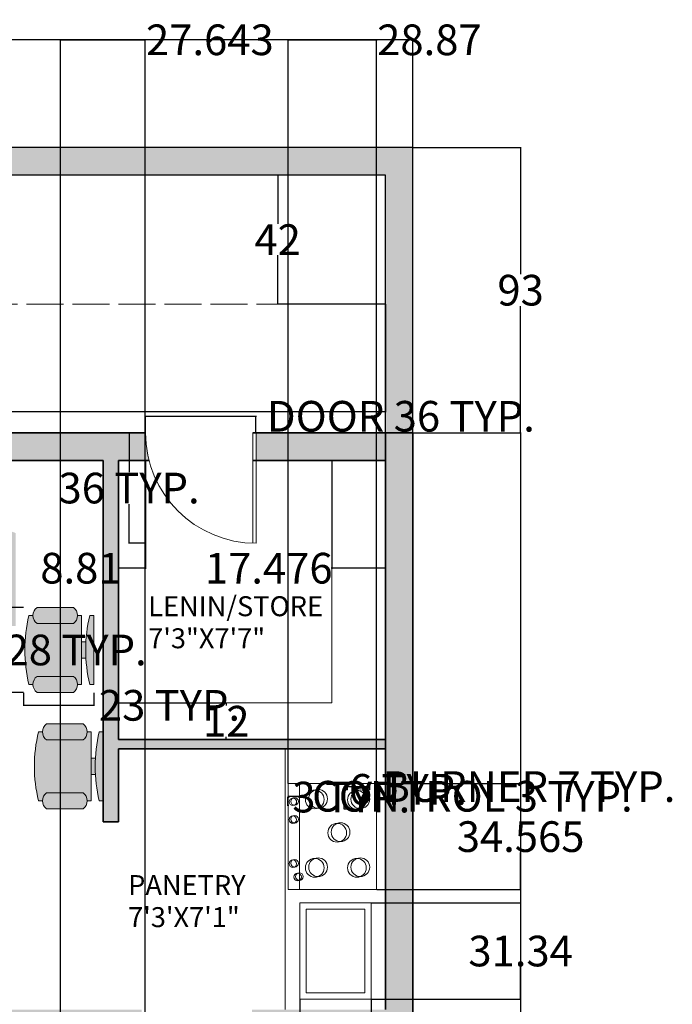
# Model space of a CAD drawing. Units: inches. Extents: x 409 to 1056, y 160 to 945.
# Tile 6 of 6: x 843 to 1056, y 624 to 945. Entities that reach past the tile are written whole.
import ezdxf

# ---------------------------------------------------------------- set-up
doc = ezdxf.new("R2010")
doc.units = ezdxf.units.IN
doc.header["$MEASUREMENT"] = 0
doc.linetypes.add('ACAD_ISO02W100', pattern=[15, 12, -3])
for name, color, linetype, lineweight in [('A-ANNO-DIMS', 2, 'Continuous', 18), ('A-AREA-IDEN', 7, 'Continuous', 18), ('A-DOOR', 3, 'Continuous', 18), ('A-EQPM', 8, 'Continuous', 18), ('A-FLOR-CASE', 8, 'Continuous', 20), ('A-FLOR-FIXT', 8, 'Continuous', 18), ('A-FURN', 8, 'Continuous', 18), ('A-ROOF-BYND', 8, 'ACAD_ISO02W100', 13), ('A-WALL', 7, 'Continuous', 35), ('A-WALL-PRPT', 7, 'Continuous', 30)]:
    doc.layers.add(name, color=color, linetype=linetype, lineweight=lineweight)
doc.layers.add('A-FURN-PATT', color=51, linetype='Continuous', lineweight=13, true_color=0xf8f6b0)
doc.layers.add('A-WALL-PATT', color=251, linetype='Continuous', lineweight=13, true_color=0x636466)
doc.styles.get("Standard").update_dxf_attribs({"font": 'arial.ttf'})
doc.dimstyles.get("Standard").update_dxf_attribs({"dimtxt": 10, "dimasz": 0.18, "dimexe": 0.18, "dimexo": 0.0625, "dimgap": 0.09, "dimtad": 0, "dimtih": 1, "dimtoh": 1, "dimdec": 0, "dimzin": 0, "dimdsep": 46, "dimlunit": 3, "dimtxsty": 'Standard', "dimcen": 0.09, "dimadec": 0, "dimazin": 0, "dimtfac": 1, "dimtdec": 0, "dimtofl": 0, "dimtmove": 0, "dimatfit": 3, "dimfxl": 1, "dimtolj": 1, "dimtzin": 0, "dimarcsym": 0})

# ---------------------------------------------------------------- blocks, each defined once
blk = doc.blocks.new('Chair - Desk')
for p, q in [((-8.5, 0), (-8.5, -1)), ((-8.5, 0), (8.5, 0)), ((8.5, 0), (8.5, -1)), ((-2, -3), (-2, -1.9355)), ((2, -1.9576), (2, -3)), ((-8.5, -3), (-8.5, -4)), ((-8.5, -3), (8.5, -3)), ((8.5, -3), (8.5, -4)), ((-10.5, -5), (-10.5, -14)), ((-6.5, -14), (-6.5, -5)), ((6.5, -5), (6.5, -14)), ((10.5, -14), (10.5, -5)), ((-8.5, -15), (-8.5, -16)), ((8.5, -15), (8.5, -16))]:
    blk.add_line(p, q)
for centre, radius, start, end in [((0, 34.625), 36.625, 256.5803, 283.4197), ((-8.5, -6.5), 2.5, 36.8699, 143.1301), ((8.5, -6.5), 2.5, 36.8699, 143.1301), ((-8.5, -12.5), 2.5, 216.8699, 323.1301), ((8.5, -12.5), 2.5, 216.8699, 323.1301), ((0, 19.625), 36.625, 256.5803, 283.4197)]:
    blk.add_arc(centre, radius, start, end)
blk = doc.blocks.new('DOOR-SWING-36IN')
for p, q in [((35, 36), (35, 0)), ((36, 36), (36, 0))]:
    blk.add_line(p, q)
blk.add_arc((36, 36), 36, 180, 270)
blk = doc.blocks.new('COOKTOP-BURNER')
for centre in [(3.06, 3.06), (4.16, 3.26)]:
    blk.add_circle(centre, 3.06)
blk = doc.blocks.new('COOKTOP-CONTROL')
for centre in [(1.22, 1.22), (1.79, 1.36)]:
    blk.add_circle(centre, 1.22)
blk = doc.blocks.new('*D11')
at = {"layer": 'A-ANNO-DIMS', "color": 0, "lineweight": -2, "transparency": 16777216}
for p, q in [((884.55, 810.81), (884.55, 816.32)), ((884.73, 816.14), (920.37, 816.14)), ((920.55, 810.81), (920.55, 816.32)), ((920.55, 816.14), (920.73, 816.14))]:
    blk.add_line(p, q, dxfattribs=at)
at = {"layer": 'A-ANNO-DIMS', "color": 0, "transparency": 16777216}
for points in [[(884.73, 816.17), (884.73, 816.11), (884.55, 816.14)], [(920.37, 816.17), (920.37, 816.11), (920.55, 816.14)]]:
    blk.add_solid(points, dxfattribs=at)
at = {"layer": 'Defpoints', "color": 0, "transparency": 16777216}
for p in [(920.55, 816.14), (884.55, 810.74), (920.55, 810.74)]:
    blk.add_point(p, dxfattribs=at)
at = {"layer": 'A-ANNO-DIMS', "color": 0, "transparency": 16777216, "insert": (967.81, 816.14), "char_height": 10, "attachment_point": 5}
blk.add_mtext('\\A1;DOOR 36 TYP.', dxfattribs=at)
blk = doc.blocks.new('*D12')
at = {"layer": 'A-ANNO-DIMS', "color": 0, "lineweight": -2, "transparency": 16777216}
for p, q in [((884.49, 810.74), (878.97, 810.74)), ((879.15, 810.56), (879.15, 797.94)), ((879.15, 774.92), (879.15, 787.54)), ((884.49, 774.74), (878.97, 774.74))]:
    blk.add_line(p, q, dxfattribs=at)
at = {"layer": 'A-ANNO-DIMS', "color": 0, "transparency": 16777216}
for points in [[(879.12, 810.56), (879.18, 810.56), (879.15, 810.74)], [(879.12, 774.92), (879.18, 774.92), (879.15, 774.74)]]:
    blk.add_solid(points, dxfattribs=at)
at = {"layer": 'Defpoints', "color": 0, "transparency": 16777216}
for p in [(879.15, 810.74), (884.55, 810.74), (884.55, 774.74)]:
    blk.add_point(p, dxfattribs=at)
at = {"layer": 'A-ANNO-DIMS', "color": 0, "transparency": 16777216, "insert": (879.15, 792.74), "char_height": 10, "attachment_point": 5}
blk.add_mtext('\\A1;36 TYP.', dxfattribs=at)
blk = doc.blocks.new('*D19')
at = {"layer": 'A-ANNO-DIMS', "color": 0, "lineweight": -2, "transparency": 16777216}
for p, q in [((844.66, 753.84), (840.37, 753.84)), ((840.55, 753.66), (840.55, 745.22)), ((840.55, 726.25), (840.55, 734.7)), ((844.66, 726.07), (840.37, 726.07))]:
    blk.add_line(p, q, dxfattribs=at)
at = {"layer": 'A-ANNO-DIMS', "color": 0, "transparency": 16777216}
for points in [[(840.52, 753.66), (840.58, 753.66), (840.55, 753.84)], [(840.52, 726.25), (840.58, 726.25), (840.55, 726.07)]]:
    blk.add_solid(points, dxfattribs=at)
at = {"layer": 'Defpoints', "color": 0, "transparency": 16777216}
for p in [(844.72, 753.84), (840.55, 726.07), (844.72, 726.07)]:
    blk.add_point(p, dxfattribs=at)
at = {"layer": 'A-ANNO-DIMS', "color": 0, "transparency": 16777216, "insert": (840.55, 739.96), "char_height": 10, "attachment_point": 5}
blk.add_mtext('\\A1;CHAIR 28 TYP.', dxfattribs=at)
blk = doc.blocks.new('*D20')
at = {"layer": 'A-ANNO-DIMS', "color": 0, "lineweight": -2, "transparency": 16777216}
for p, q in [((844.72, 726.01), (844.72, 721.73)), ((867.64, 726.01), (867.64, 721.73)), ((844.9, 721.91), (867.46, 721.91)), ((867.64, 721.91), (867.82, 721.91))]:
    blk.add_line(p, q, dxfattribs=at)
at = {"layer": 'A-ANNO-DIMS', "color": 0, "transparency": 16777216}
for points in [[(844.9, 721.94), (844.9, 721.88), (844.72, 721.91)], [(867.46, 721.94), (867.46, 721.88), (867.64, 721.91)]]:
    blk.add_solid(points, dxfattribs=at)
at = {"layer": 'Defpoints', "color": 0, "transparency": 16777216}
for p in [(844.72, 726.07), (867.64, 726.07), (867.64, 721.91)]:
    blk.add_point(p, dxfattribs=at)
at = {"layer": 'A-ANNO-DIMS', "color": 0, "transparency": 16777216, "insert": (892.33, 721.91), "char_height": 10, "attachment_point": 5}
blk.add_mtext('\\A1;23 TYP.', dxfattribs=at)
blk = doc.blocks.new('*D31')
at = {"layer": 'A-ANNO-DIMS', "color": 0, "lineweight": -2, "transparency": 16777216}
for p, q in [((950.42, 694.4), (950.42, 695.6)), ((950.6, 695.42), (957.46, 695.42)), ((957.64, 694.4), (957.64, 695.6)), ((957.64, 695.42), (957.82, 695.42))]:
    blk.add_line(p, q, dxfattribs=at)
at = {"layer": 'A-ANNO-DIMS', "color": 0, "transparency": 16777216}
for points in [[(950.6, 695.45), (950.6, 695.39), (950.42, 695.42)], [(957.46, 695.45), (957.46, 695.39), (957.64, 695.42)]]:
    blk.add_solid(points, dxfattribs=at)
at = {"layer": 'Defpoints', "color": 0, "transparency": 16777216}
for p in [(950.42, 694.34), (957.64, 695.42), (957.64, 694.34)]:
    blk.add_point(p, dxfattribs=at)
at = {"layer": 'A-ANNO-DIMS', "color": 0, "transparency": 16777216, "insert": (1009.57, 695.42), "char_height": 10, "attachment_point": 5}
blk.add_mtext('\\A1;BURNER 7 TYP.', dxfattribs=at)
blk = doc.blocks.new('*D32')
at = {"layer": 'A-ANNO-DIMS', "color": 0, "lineweight": -2, "transparency": 16777216}
for p, q in [((950.35, 694.34), (949.15, 694.34)), ((949.33, 694.34), (949.33, 694.52)), ((949.33, 694.52), (949.51, 694.52)), ((949.33, 688.2), (949.33, 694.16)), ((950.35, 688.02), (949.15, 688.02))]:
    blk.add_line(p, q, dxfattribs=at)
at = {"layer": 'A-ANNO-DIMS', "color": 0, "transparency": 16777216}
for points in [[(949.3, 694.16), (949.36, 694.16), (949.33, 694.34)], [(949.3, 688.2), (949.36, 688.2), (949.33, 688.02)]]:
    blk.add_solid(points, dxfattribs=at)
at = {"layer": 'Defpoints', "color": 0, "transparency": 16777216}
for p in [(949.33, 694.34), (950.42, 694.34), (950.42, 688.02)]:
    blk.add_point(p, dxfattribs=at)
at = {"layer": 'A-ANNO-DIMS', "color": 0, "transparency": 16777216, "insert": (970.08, 694.52), "char_height": 10, "attachment_point": 5}
blk.add_mtext('\\A1;6 TYP.', dxfattribs=at)
blk = doc.blocks.new('*D33')
at = {"layer": 'A-ANNO-DIMS', "color": 0, "lineweight": -2, "transparency": 16777216}
for p, q in [((931.36, 691.88), (931.36, 692.45)), ((931.54, 692.27), (934.2, 692.27)), ((934.38, 691.88), (934.38, 692.45)), ((934.38, 692.27), (934.56, 692.27))]:
    blk.add_line(p, q, dxfattribs=at)
at = {"layer": 'A-ANNO-DIMS', "color": 0, "transparency": 16777216}
for points in [[(931.54, 692.3), (931.54, 692.24), (931.36, 692.27)], [(934.2, 692.3), (934.2, 692.24), (934.38, 692.27)]]:
    blk.add_solid(points, dxfattribs=at)
at = {"layer": 'Defpoints', "color": 0, "transparency": 16777216}
for p in [(931.36, 691.82), (934.38, 692.27), (934.38, 691.82)]:
    blk.add_point(p, dxfattribs=at)
at = {"layer": 'A-ANNO-DIMS', "color": 0, "transparency": 16777216, "insert": (991.14, 692.27), "char_height": 10, "attachment_point": 5}
blk.add_mtext('\\A1;CONTROL 3 TYP.', dxfattribs=at)
blk = doc.blocks.new('*D34')
at = {"layer": 'A-ANNO-DIMS', "color": 0, "lineweight": -2, "transparency": 16777216}
for p, q in [((931.3, 691.82), (930.73, 691.82)), ((930.91, 691.82), (930.91, 692)), ((930.91, 692), (931.09, 692)), ((930.91, 689.41), (930.91, 691.64)), ((931.3, 689.23), (930.73, 689.23))]:
    blk.add_line(p, q, dxfattribs=at)
at = {"layer": 'A-ANNO-DIMS', "color": 0, "transparency": 16777216}
for points in [[(930.88, 691.64), (930.94, 691.64), (930.91, 691.82)], [(930.88, 689.41), (930.94, 689.41), (930.91, 689.23)]]:
    blk.add_solid(points, dxfattribs=at)
at = {"layer": 'Defpoints', "color": 0, "transparency": 16777216}
for p in [(930.91, 691.82), (931.36, 691.82), (931.36, 689.23)]:
    blk.add_point(p, dxfattribs=at)
at = {"layer": 'A-ANNO-DIMS', "color": 0, "transparency": 16777216, "insert": (951.63, 692), "char_height": 10, "attachment_point": 5}
blk.add_mtext('\\A1;3 TYP.', dxfattribs=at)
blk = doc.blocks.new('*D35')
at = {"layer": 'A-ANNO-DIMS', "color": 0, "lineweight": -2, "transparency": 16777216}
for p, q in [((455.74, 903.81), (455.74, 939.05)), ((455.92, 938.87), (702.61, 938.87)), ((971.56, 938.87), (724.88, 938.87)), ((971.74, 903.81), (971.74, 939.05))]:
    blk.add_line(p, q, dxfattribs=at)
at = {"layer": 'A-ANNO-DIMS', "color": 0, "transparency": 16777216}
for points in [[(455.92, 938.9), (455.92, 938.84), (455.74, 938.87)], [(971.56, 938.9), (971.56, 938.84), (971.74, 938.87)]]:
    blk.add_solid(points, dxfattribs=at)
at = {"layer": 'Defpoints', "color": 0, "transparency": 16777216}
for p in [(971.74, 938.87), (455.74, 903.74), (971.74, 903.74)]:
    blk.add_point(p, dxfattribs=at)
at = {"layer": 'A-ANNO-DIMS', "color": 0, "transparency": 16777216, "insert": (713.74, 938.87), "char_height": 10, "attachment_point": 5}
blk.add_mtext('\\A1;516', dxfattribs=at)
blk = doc.blocks.new('*D38')
at = {"layer": 'A-ANNO-DIMS', "color": 0, "lineweight": -2, "transparency": 16777216}
for p, q in [((971.8, 810.74), (1007.05, 810.74)), ((1006.87, 810.56), (1006.87, 530.94)), ((1006.87, 240.92), (1006.87, 520.55)), ((971.8, 240.74), (1007.05, 240.74))]:
    blk.add_line(p, q, dxfattribs=at)
at = {"layer": 'A-ANNO-DIMS', "color": 0, "transparency": 16777216}
for points in [[(1006.84, 810.56), (1006.9, 810.56), (1006.87, 810.74)], [(1006.84, 240.92), (1006.9, 240.92), (1006.87, 240.74)]]:
    blk.add_solid(points, dxfattribs=at)
at = {"layer": 'Defpoints', "color": 0, "transparency": 16777216}
for p in [(971.74, 810.74), (1006.87, 810.74), (971.74, 240.74)]:
    blk.add_point(p, dxfattribs=at)
at = {"layer": 'A-ANNO-DIMS', "color": 0, "transparency": 16777216, "insert": (1006.87, 525.74), "char_height": 10, "attachment_point": 5}
blk.add_mtext('\\A1;570', dxfattribs=at)
blk = doc.blocks.new('*D41')
at = {"layer": 'A-ANNO-DIMS', "color": 0, "lineweight": -2, "transparency": 16777216}
for p, q in [((934.87, 626.08), (934.87, 166.44)), ((958.09, 626.08), (958.09, 166.44)), ((935.05, 166.62), (957.91, 166.62)), ((958.09, 166.62), (958.27, 166.62))]:
    blk.add_line(p, q, dxfattribs=at)
at = {"layer": 'A-ANNO-DIMS', "color": 0, "transparency": 16777216}
for points in [[(935.05, 166.65), (935.05, 166.59), (934.87, 166.62)], [(957.91, 166.65), (957.91, 166.59), (958.09, 166.62)]]:
    blk.add_solid(points, dxfattribs=at)
at = {"layer": 'Defpoints', "color": 0, "transparency": 16777216}
for p in [(934.87, 626.14), (958.09, 626.14), (958.09, 166.62)]:
    blk.add_point(p, dxfattribs=at)
at = {"layer": 'A-ANNO-DIMS', "color": 0, "transparency": 16777216, "insert": (975.27, 166.62), "char_height": 10, "attachment_point": 5}
blk.add_mtext('\\A1;23.22', dxfattribs=at)
blk = doc.blocks.new('*D42')
at = {"layer": 'A-ANNO-DIMS', "color": 0, "lineweight": -2, "transparency": 16777216}
for p, q in [((958.15, 657.48), (1007.05, 657.48)), ((1006.87, 657.3), (1006.87, 647.01)), ((1006.87, 626.32), (1006.87, 636.61)), ((958.15, 626.14), (1007.05, 626.14))]:
    blk.add_line(p, q, dxfattribs=at)
at = {"layer": 'A-ANNO-DIMS', "color": 0, "transparency": 16777216}
for points in [[(1006.84, 657.3), (1006.9, 657.3), (1006.87, 657.48)], [(1006.84, 626.32), (1006.9, 626.32), (1006.87, 626.14)]]:
    blk.add_solid(points, dxfattribs=at)
at = {"layer": 'Defpoints', "color": 0, "transparency": 16777216}
for p in [(958.09, 657.48), (1006.87, 657.48), (958.09, 626.14)]:
    blk.add_point(p, dxfattribs=at)
at = {"layer": 'A-ANNO-DIMS', "color": 0, "transparency": 16777216, "insert": (1006.87, 641.81), "char_height": 10, "attachment_point": 5}
blk.add_mtext('\\A1;31.34', dxfattribs=at)
blk = doc.blocks.new('*D43')
at = {"layer": 'A-ANNO-DIMS', "color": 0, "lineweight": -2, "transparency": 16777216}
for p, q in [((931.02, 696.45), (931.02, 939.05)), ((931.2, 938.87), (959.71, 938.87)), ((959.89, 696.45), (959.89, 939.05)), ((959.89, 938.87), (960.07, 938.87))]:
    blk.add_line(p, q, dxfattribs=at)
at = {"layer": 'A-ANNO-DIMS', "color": 0, "transparency": 16777216}
for points in [[(931.2, 938.9), (931.2, 938.84), (931.02, 938.87)], [(959.71, 938.9), (959.71, 938.84), (959.89, 938.87)]]:
    blk.add_solid(points, dxfattribs=at)
at = {"layer": 'Defpoints', "color": 0, "transparency": 16777216}
for p in [(959.89, 938.87), (931.02, 696.39), (959.89, 696.39)]:
    blk.add_point(p, dxfattribs=at)
at = {"layer": 'A-ANNO-DIMS', "color": 0, "transparency": 16777216, "insert": (977.12, 938.87), "char_height": 10, "attachment_point": 5}
blk.add_mtext('\\A1;28.87', dxfattribs=at)
blk = doc.blocks.new('*D44')
at = {"layer": 'A-ANNO-DIMS', "color": 0, "lineweight": -2, "transparency": 16777216}
for p, q in [((959.95, 696.39), (1007.05, 696.39)), ((1006.87, 696.21), (1006.87, 684.31)), ((1006.87, 662), (1006.87, 673.91)), ((959.95, 661.82), (1007.05, 661.82))]:
    blk.add_line(p, q, dxfattribs=at)
at = {"layer": 'A-ANNO-DIMS', "color": 0, "transparency": 16777216}
for points in [[(1006.84, 696.21), (1006.9, 696.21), (1006.87, 696.39)], [(1006.84, 662), (1006.9, 662), (1006.87, 661.82)]]:
    blk.add_solid(points, dxfattribs=at)
at = {"layer": 'Defpoints', "color": 0, "transparency": 16777216}
for p in [(959.89, 696.39), (1006.87, 696.39), (959.89, 661.82)]:
    blk.add_point(p, dxfattribs=at)
at = {"layer": 'A-ANNO-DIMS', "color": 0, "transparency": 16777216, "insert": (1006.87, 679.11), "char_height": 10, "attachment_point": 5}
blk.add_mtext('\\A1;34.565', dxfattribs=at)
blk = doc.blocks.new('*D51')
at = {"layer": 'A-ANNO-DIMS', "color": 0, "lineweight": -2, "transparency": 16777216}
for p, q in [((856.74, 613.81), (856.74, 939.05)), ((856.92, 938.87), (884.2, 938.87)), ((884.38, 613.81), (884.38, 939.05)), ((884.38, 938.87), (884.56, 938.87))]:
    blk.add_line(p, q, dxfattribs=at)
at = {"layer": 'A-ANNO-DIMS', "color": 0, "transparency": 16777216}
for points in [[(856.92, 938.9), (856.92, 938.84), (856.74, 938.87)], [(884.2, 938.9), (884.2, 938.84), (884.38, 938.87)]]:
    blk.add_solid(points, dxfattribs=at)
at = {"layer": 'Defpoints', "color": 0, "transparency": 16777216}
for p in [(884.38, 938.87), (856.74, 613.74), (884.38, 613.74)]:
    blk.add_point(p, dxfattribs=at)
at = {"layer": 'A-ANNO-DIMS', "color": 0, "transparency": 16777216, "insert": (905.5, 938.87), "char_height": 10, "attachment_point": 5}
blk.add_mtext('\\A1;27.643', dxfattribs=at)
blk = doc.blocks.new('*D57')
at = {"layer": 'A-ANNO-DIMS', "color": 0, "lineweight": -2, "transparency": 16777216}
for p, q in [((875.74, 801.68), (875.74, 766.44)), ((884.55, 801.68), (884.55, 766.44)), ((875.74, 766.62), (875.56, 766.62)), ((884.37, 766.62), (875.92, 766.62))]:
    blk.add_line(p, q, dxfattribs=at)
at = {"layer": 'A-ANNO-DIMS', "color": 0, "transparency": 16777216}
for points in [[(875.92, 766.65), (875.92, 766.59), (875.74, 766.62)], [(884.37, 766.65), (884.37, 766.59), (884.55, 766.62)]]:
    blk.add_solid(points, dxfattribs=at)
at = {"layer": 'Defpoints', "color": 0, "transparency": 16777216}
for p in [(875.74, 801.74), (884.55, 801.74), (875.74, 766.62)]:
    blk.add_point(p, dxfattribs=at)
at = {"layer": 'A-ANNO-DIMS', "color": 0, "transparency": 16777216, "insert": (863.44, 766.62), "char_height": 10, "attachment_point": 5}
blk.add_mtext('\\A1;8.81', dxfattribs=at)
blk = doc.blocks.new('*D59')
at = {"layer": 'A-ANNO-DIMS', "color": 0, "lineweight": -2, "transparency": 16777216}
for p, q in [((971.8, 903.74), (1007.05, 903.74)), ((1006.87, 903.56), (1006.87, 862.44)), ((1006.87, 810.92), (1006.87, 852.04)), ((971.8, 810.74), (1007.05, 810.74))]:
    blk.add_line(p, q, dxfattribs=at)
at = {"layer": 'A-ANNO-DIMS', "color": 0, "transparency": 16777216}
for points in [[(1006.84, 903.56), (1006.9, 903.56), (1006.87, 903.74)], [(1006.84, 810.92), (1006.9, 810.92), (1006.87, 810.74)]]:
    blk.add_solid(points, dxfattribs=at)
at = {"layer": 'Defpoints', "color": 0, "transparency": 16777216}
for p in [(971.74, 903.74), (1006.87, 903.74), (971.74, 810.74)]:
    blk.add_point(p, dxfattribs=at)
at = {"layer": 'A-ANNO-DIMS', "color": 0, "transparency": 16777216, "insert": (1006.87, 857.24), "char_height": 10, "attachment_point": 5}
blk.add_mtext('\\A1;93', dxfattribs=at)
blk = doc.blocks.new('*D60')
at = {"layer": 'A-ANNO-DIMS', "color": 0, "lineweight": -2, "transparency": 16777216}
for p, q in [((537.3, 852.68), (537.3, 817.44)), ((962.74, 852.68), (962.74, 817.44)), ((537.48, 817.62), (728.99, 817.62)), ((962.56, 817.62), (771.05, 817.62))]:
    blk.add_line(p, q, dxfattribs=at)
at = {"layer": 'A-ANNO-DIMS', "color": 0, "transparency": 16777216}
for points in [[(537.48, 817.65), (537.48, 817.59), (537.3, 817.62)], [(962.56, 817.65), (962.56, 817.59), (962.74, 817.62)]]:
    blk.add_solid(points, dxfattribs=at)
at = {"layer": 'Defpoints', "color": 0, "transparency": 16777216}
for p in [(537.3, 852.74), (962.74, 852.74), (537.3, 817.62)]:
    blk.add_point(p, dxfattribs=at)
at = {"layer": 'A-ANNO-DIMS', "color": 0, "transparency": 16777216, "insert": (750.02, 817.62), "char_height": 10, "attachment_point": 5}
blk.add_mtext('\\A1;425.44', dxfattribs=at)
blk = doc.blocks.new('*D61')
at = {"layer": 'A-ANNO-DIMS', "color": 0, "lineweight": -2, "transparency": 16777216}
for p, q in [((962.68, 894.74), (927.44, 894.74)), ((927.62, 894.56), (927.62, 878.85)), ((927.62, 852.92), (927.62, 868.63)), ((962.68, 852.74), (927.44, 852.74))]:
    blk.add_line(p, q, dxfattribs=at)
at = {"layer": 'A-ANNO-DIMS', "color": 0, "transparency": 16777216}
for points in [[(927.59, 894.56), (927.65, 894.56), (927.62, 894.74)], [(927.59, 852.92), (927.65, 852.92), (927.62, 852.74)]]:
    blk.add_solid(points, dxfattribs=at)
at = {"layer": 'Defpoints', "color": 0, "transparency": 16777216}
for p in [(927.62, 894.74), (962.74, 894.74), (962.74, 852.74)]:
    blk.add_point(p, dxfattribs=at)
at = {"layer": 'A-ANNO-DIMS', "color": 0, "transparency": 16777216, "insert": (927.62, 873.74), "char_height": 10, "attachment_point": 5}
blk.add_mtext('\\A1;42', dxfattribs=at)
blk = doc.blocks.new('*D64')
at = {"layer": 'A-ANNO-DIMS', "color": 0, "lineweight": -2, "transparency": 16777216}
for p, q in [((945.27, 801.68), (945.27, 766.44)), ((962.74, 801.68), (962.74, 766.44)), ((945.27, 766.62), (945.09, 766.62)), ((962.56, 766.62), (945.45, 766.62))]:
    blk.add_line(p, q, dxfattribs=at)
at = {"layer": 'A-ANNO-DIMS', "color": 0, "transparency": 16777216}
for points in [[(945.45, 766.65), (945.45, 766.59), (945.27, 766.62)], [(962.56, 766.65), (962.56, 766.59), (962.74, 766.62)]]:
    blk.add_solid(points, dxfattribs=at)
at = {"layer": 'Defpoints', "color": 0, "transparency": 16777216}
for p in [(945.27, 801.74), (962.74, 801.74), (945.27, 766.62)]:
    blk.add_point(p, dxfattribs=at)
at = {"layer": 'A-ANNO-DIMS', "color": 0, "transparency": 16777216, "insert": (924.71, 766.62), "char_height": 10, "attachment_point": 5}
blk.add_mtext('\\A1;17.476', dxfattribs=at)
blk = doc.blocks.new('*D65')
at = {"layer": 'A-ANNO-DIMS', "color": 0, "lineweight": -2, "transparency": 16777216}
for p, q in [((875.8, 722.74), (911.05, 722.74)), ((910.87, 722.56), (910.87, 721.85)), ((875.8, 710.74), (911.05, 710.74)), ((910.87, 710.92), (910.87, 711.63))]:
    blk.add_line(p, q, dxfattribs=at)
at = {"layer": 'A-ANNO-DIMS', "color": 0, "transparency": 16777216}
for points in [[(910.84, 722.56), (910.9, 722.56), (910.87, 722.74)], [(910.84, 710.92), (910.9, 710.92), (910.87, 710.74)]]:
    blk.add_solid(points, dxfattribs=at)
at = {"layer": 'Defpoints', "color": 0, "transparency": 16777216}
for p in [(875.74, 722.74), (875.74, 710.74), (910.87, 710.74)]:
    blk.add_point(p, dxfattribs=at)
at = {"layer": 'A-ANNO-DIMS', "color": 0, "transparency": 16777216, "insert": (910.87, 716.74), "char_height": 10, "attachment_point": 5}
blk.add_mtext('\\A1;12', dxfattribs=at)

msp = doc.modelspace()

# ---------------------------------------------------------------- hatches: boundary and pattern name
at = {"layer": 'A-FURN-PATT', "transparency": 33554661}
h = msp.add_hatch(color=256, dxfattribs=at)
h.dxf.hatch_style = 1
h.paths.add_polyline_path([(700.0326, 771.7872), (672.0783, 771.7872), (672.0783, 749.5866), (700.0326, 749.5866)], flags=17)
h.paths.add_polyline_path([(727.9869, 771.7872), (700.0326, 771.7872), (700.0326, 749.5866), (727.9869, 749.5866)], flags=17)
h.paths.add_polyline_path([(700.0326, 779.6917), (700.0326, 771.7872), (727.9869, 771.7872), (727.9869, 774.0139, 0.05064665)], flags=17)
h.paths.add_polyline_path([(700.0326, 779.6917, 0.04962821), (672.0783, 779.6917), (672.0783, 771.7872), (700.0326, 771.7872)], flags=17)
h.paths.add_polyline_path([(672.0783, 779.6917, 0.05064665), (644.124, 774.0139), (644.124, 771.7872), (672.0783, 771.7872)], flags=17)
h.paths.add_polyline_path([(672.0783, 771.7872), (644.124, 771.7872), (644.124, 749.5866), (672.0783, 749.5866)], flags=17)
h.paths.add_polyline_path([(637.1355, 778.0558), (637.1355, 747.772), (644.124, 747.772), (644.124, 774.0139, -0.15194781), (727.9869, 774.0139), (727.9869, 771.7872), (727.9869, 749.5866), (727.9869, 747.772), (734.9755, 747.772), (734.9755, 778.0558, 0.19047621)])
h.paths.add_polyline_path([(751.3563, 774.0139, -0.15194781), (835.2192, 774.0139), (835.2192, 747.772), (842.2077, 747.772), (842.2077, 778.0558, 0.19047621), (744.3677, 778.0558), (744.3677, 747.772), (751.3563, 747.772)])
h.paths.add_polyline_path([(779.3105, 771.7872), (751.3563, 771.7872), (751.3563, 749.5866), (779.3106, 749.5866)], flags=17)
h.paths.add_polyline_path([(807.2649, 771.7872), (779.3105, 771.7872), (779.3106, 749.5866), (807.2648, 749.5866)], flags=17)
h.paths.add_polyline_path([(835.2192, 771.7872), (807.2649, 771.7872), (807.2648, 749.5866), (835.2192, 749.5866)], flags=17)
h.paths.add_polyline_path([(835.2192, 774.0139, 0.05064665), (807.2649, 779.6917), (807.2649, 771.7872), (835.2192, 771.7872)], flags=17)
h.paths.add_polyline_path([(807.2649, 779.6917, 0.04962821), (779.3105, 779.6917), (779.3105, 771.7872), (807.2649, 771.7872)], flags=17)
h.paths.add_polyline_path([(779.3105, 779.6917, 0.05064665), (751.3563, 774.0139), (751.3563, 771.7872), (779.3105, 771.7872)], flags=17)
h.paths.add_polyline_path([(863.6721, 751.196), (862.3498, 751.196, -0.23606798), (861.0276, 748.5515), (849.1271, 748.5515, -0.23606798), (847.8048, 751.196), (846.4825, 751.196, 0.11764706), (846.4825, 728.7174), (847.8048, 728.7174, -0.23606798), (849.1271, 731.3619), (861.0276, 731.3619, -0.23606798), (862.3498, 728.7174), (863.6721, 728.7174)])
h.paths.add_polyline_path([(861.0276, 753.8406), (849.1271, 753.8406, 0.5), (849.1271, 748.5515), (861.0276, 748.5515, 0.23606798), (862.3498, 751.196, 0.23606798)])
h.paths.add_polyline_path([(861.0276, 731.3619), (849.1271, 731.3619, 0.23606798), (847.8048, 728.7174, 0.23606798), (849.1271, 726.0728), (861.0276, 726.0728, 0.5)])
h.paths.add_polyline_path([(867.6389, 751.196), (866.3167, 751.196, 0.11764706), (866.3167, 728.7174), (867.6389, 728.7174)])
h.paths.add_polyline_path([(865.0666, 742.6012), (863.6721, 742.6012), (863.6721, 737.3121), (865.0666, 737.3121, -0.02732414)])
h.paths.add_polyline_path([(864.1304, 715.9038), (852.2299, 715.9038, 0.5), (852.2299, 710.6147), (864.1304, 710.6147, 0.5)])
h.paths.add_polyline_path([(866.7749, 713.2593), (865.4527, 713.2593, -0.23606798), (864.1304, 710.6147), (852.2299, 710.6147, -0.23606798), (850.9076, 713.2593), (849.5854, 713.2593, 0.11764706), (849.5854, 690.7806), (850.9076, 690.7806, -0.23606798), (852.2299, 693.4252), (864.1304, 693.4252, -0.23606798), (865.4527, 690.7806), (866.7749, 690.7806)])
h.paths.add_polyline_path([(864.1304, 693.4252), (852.2299, 693.4252, 0.5), (852.2299, 688.1361), (864.1304, 688.1361, 0.5)])
h.paths.add_polyline_path([(868.1695, 704.6645), (866.7749, 704.6645), (866.7749, 699.3754), (868.1695, 699.3754, -0.02732414)])
h.paths.add_polyline_path([(870.7418, 713.2593), (869.4195, 713.2593, 0.11764706), (869.4195, 690.7806), (870.7418, 690.7806)])
h.paths.add_polyline_path([(796.1541, 700.7668), (803.8768, 698.1956), (796.8278, 694.1258, 4.66316556)])
h.paths.add_polyline_path([(722.7253, 700.7668), (730.4481, 698.1956), (723.399, 694.1258, 4.66316556)])
h.paths.add_polyline_path([(669.7198, 709.3627), (668.8708, 710.3764, -0.23606798), (665.9944, 709.692), (658.3533, 718.8153, -0.23606798), (659.5316, 721.527), (658.6826, 722.5407), (641.4498, 708.1074), (642.2988, 707.0937, -0.23606798), (645.1752, 707.7781), (652.8164, 698.6548, -0.23606798), (651.638, 695.9431), (652.487, 694.9294, 0.11764706)])
h.paths.add_polyline_path([(645.1752, 707.7781, 0.5), (641.1204, 704.382), (648.7616, 695.2587, 0.5), (652.8164, 698.6548)])
h.paths.add_polyline_path([(662.4081, 722.2113, 0.5), (658.3533, 718.8153), (665.9944, 709.692, 0.23606798), (668.8708, 710.3764, 0.23606798), (670.0492, 713.0881)])
h.paths.add_polyline_path([(656.9846, 724.5681), (656.1356, 725.5818), (638.9027, 711.1485), (639.7518, 710.1348, 0.11764706)])
h.paths.add_polyline_path([(652.0936, 717.0221), (651.1982, 718.0912, -0.02732414), (647.1434, 714.6951), (648.0388, 713.626)], flags=17)
at = {"layer": 'A-WALL-PATT'}
h = msp.add_hatch(color=256, dxfattribs=at)
h.dxf.hatch_style = 1
h.paths.add_polyline_path([(730.4481, 698.1956), (696.9841, 709.3369, 1), (696.9841, 678.8752)], flags=17)
h.paths.add_polyline_path([(803.8768, 698.1956), (770.4128, 709.3369, 1), (770.4128, 678.8752)], flags=17)
h.paths.add_polyline_path([(464.7418, 894.7439), (466.7418, 894.7439), (962.7418, 894.7439), (962.7418, 810.7439), (971.7418, 810.7439), (971.7418, 903.7439), (455.7418, 903.7439), (455.7418, 201.7439), (971.7418, 201.7439), (971.7418, 240.7439), (962.7418, 240.7439), (962.7418, 210.7439), (464.7418, 210.7439)])
h = msp.add_hatch(color=256, dxfattribs=at)
h.dxf.hatch_style = 1
h.paths.add_polyline_path([(626.7418, 801.7439), (870.7418, 801.7439), (870.7418, 710.7439), (870.7418, 683.9043), (875.7418, 683.9043), (875.7418, 707.7439), (962.7418, 707.7439), (962.7418, 710.7439), (875.7418, 710.7439), (875.7418, 722.7439), (875.7418, 801.7439), (885.6955, 801.7439, -0.06325422), (884.5523, 810.7439), (617.7418, 810.7439), (617.7418, 732.9297), (626.7418, 732.9297)])
h.paths.add_polyline_path([(962.7418, 810.7439), (920.5523, 810.7439), (920.5523, 801.7439), (962.7418, 801.7439)], flags=17)
h.paths.add_polyline_path([(971.7418, 810.7439), (962.7418, 810.7439), (962.7418, 801.7439), (962.7418, 707.7439), (962.7418, 622.7439), (962.7418, 613.7439), (962.7418, 548.7439), (856.7418, 548.7439), (847.7418, 548.7439), (776.7418, 548.7439), (776.7418, 569.8172), (768.7418, 569.8172), (768.7418, 539.7439), (847.7418, 539.7439), (971.7418, 539.7439), (971.7418, 613.7439), (971.7418, 707.7439)])
h.paths.add_polyline_path([(883.2418, 622.7439), (875.7418, 622.7439), (684.4993, 622.7439, -0.06325422), (685.6424, 613.7439), (870.7418, 613.7439), (875.7418, 613.7439), (884.3849, 613.7439, -0.06325422)])
h.paths.add_polyline_path([(649.6424, 622.7439), (626.7418, 622.7439), (626.7418, 613.7439), (649.6424, 613.7439)])
h.paths.add_polyline_path([(626.7418, 652.3165), (617.7418, 652.3165), (617.7418, 613.7439), (626.7418, 613.7439), (626.7418, 622.7439)])
h.paths.add_polyline_path([(776.7418, 613.7439), (768.7418, 613.7439), (768.7418, 590.4138), (776.7418, 590.4138)], flags=17)
h.paths.add_polyline_path([(856.7418, 613.7439), (847.7418, 613.7439), (847.7418, 548.7439), (856.7418, 548.7439)], flags=17)
h.paths.add_polyline_path([(962.7418, 622.7439), (919.2418, 622.7439), (919.2418, 613.7439), (962.7418, 613.7439)], flags=17)
h.paths.add_polyline_path([(971.7418, 539.7439), (962.7418, 539.7439), (962.7418, 452.7439), (687.1506, 452.7439, -0.06325422), (686.0074, 443.7439), (962.7418, 443.7439), (962.7418, 331.7439), (927.6873, 331.7439, -0.02784244), (927.9102, 327.7439), (962.7418, 327.7439), (962.7418, 249.7439), (871.7418, 249.7439), (870.7418, 249.7439), (626.7418, 249.7439), (626.7418, 282.7439), (617.7418, 282.7439), (617.7418, 240.7439), (870.7418, 240.7439), (871.7418, 240.7439), (971.7418, 240.7439), (971.7418, 249.7439), (971.7418, 327.7439), (971.7418, 331.7439), (971.7418, 443.7439), (971.7418, 452.7439)])
h.paths.add_polyline_path([(875.7418, 443.7439), (870.7418, 443.7439), (870.7418, 327.7439), (871.7418, 327.7439), (891.9102, 327.7439), (891.9102, 331.7439), (875.7418, 331.7439)], flags=17)

# ---------------------------------------------------------------- linework, layer by layer
at = {"layer": 'A-DOOR'}
for p, q in [((920.5523, 801.7439), (920.5523, 810.7439)), ((884.5523, 801.7439), (885.6955, 801.7439)), ((919.5523, 801.7439), (920.5523, 801.7439))]:
    msp.add_line(p, q, dxfattribs=at)
at = {"layer": 'A-EQPM'}
for p, q in [((931.0176, 661.8238), (931.0176, 696.3886)), ((931.0176, 696.3886), (934.7013, 696.3886)), ((934.7013, 661.8238), (931.0176, 661.8238))]:
    msp.add_line(p, q, dxfattribs=at)
msp.add_lwpolyline([(934.7013, 696.3886), (959.8882, 696.3886), (959.8882, 661.8238), (934.7013, 661.8238)], close=True, dxfattribs=at)
msp.add_circle((932.5858, 690.4505), 1.2239, dxfattribs=at)
at = {"layer": 'A-FLOR-CASE'}
for p, q in [((945.2662, 722.7439), (945.2662, 801.7439)), ((875.7418, 710.7439), (875.7418, 722.7439)), ((875.7418, 722.7439), (945.2662, 722.7439)), ((930.0665, 707.7439), (930.0665, 622.7439))]:
    msp.add_line(p, q, dxfattribs=at)
at = {"layer": 'A-FLOR-FIXT'}
for points in [[(934.8736, 657.4805), (958.0915, 657.4805), (958.0915, 626.1427), (934.8736, 626.1427)], [(936.8736, 655.4805), (956.0915, 655.4805), (956.0915, 628.1427), (936.8736, 628.1427)]]:
    msp.add_lwpolyline(points, close=True, dxfattribs=at)
at = {"layer": 'A-ROOF-BYND'}
msp.add_line((962.7418, 852.7439), (537.2978, 852.7439), dxfattribs=at)
at = {"layer": 'A-WALL'}
for p, q in [((884.5523, 810.7439), (617.7418, 810.7439)), ((884.5523, 810.7439), (875.7418, 810.7439)), ((971.7418, 810.7439), (919.5523, 810.7439)), ((971.7418, 810.7439), (919.5523, 810.7439)), ((962.7418, 801.7439), (962.7418, 810.7439)), ((971.7418, 705.7439), (971.7418, 810.7439)), ((870.7418, 801.7439), (626.7418, 801.7439)), ((870.7418, 801.7439), (870.7418, 710.7439)), ((875.7418, 801.7439), (875.7418, 710.7439)), ((885.6955, 801.7439), (875.7418, 801.7439)), ((962.7418, 801.7439), (919.5523, 801.7439)), ((962.7418, 707.7439), (962.7418, 801.7439)), ((870.7418, 683.9043), (870.7418, 710.7439)), ((875.7418, 710.7439), (962.7418, 710.7439)), ((875.7418, 707.7439), (875.7418, 683.9043)), ((875.7418, 707.7439), (962.7418, 707.7439)), ((962.7418, 707.7439), (962.7418, 622.7439)), ((971.7418, 707.7439), (971.7418, 613.7439)), ((870.7418, 683.9043), (875.7418, 683.9043))]:
    msp.add_line(p, q, dxfattribs=at)
at = {"layer": 'A-WALL-PRPT'}
for p, q in [((971.7418, 903.7439), (455.7418, 903.7439)), ((971.7418, 810.7439), (971.7418, 903.7439)), ((962.7418, 894.7439), (466.7418, 894.7439)), ((962.7418, 810.7439), (962.7418, 894.7439))]:
    msp.add_line(p, q, dxfattribs=at)

# ---------------------------------------------------------------- block references
at = {"layer": 'A-DOOR'}
msp.add_blockref('DOOR-SWING-36IN', (884.552, 774.744), dxfattribs=at)
at = {"layer": 'A-EQPM'}
for name, p in [('COOKTOP-BURNER', (936.6471, 688.1634)), ('COOKTOP-BURNER', (950.415, 688.018)), ('COOKTOP-CONTROL', (931.362, 689.227)), ('COOKTOP-CONTROL', (931.362, 683.4121)), ('COOKTOP-BURNER', (943.9771, 677.3024)), ('COOKTOP-CONTROL', (931.362, 669.06)), ('COOKTOP-BURNER', (936.6471, 665.8782)), ('COOKTOP-BURNER', (950.415, 665.8782)), ('COOKTOP-CONTROL', (932.9069, 664.7275))]:
    msp.add_blockref(name, p, dxfattribs=at)
at = {"layer": 'A-FURN', "xscale": 1.322274350512926, "yscale": 1.322274350512926, "zscale": 1.322274350512926, "rotation": 270}
for p in [(867.6389, 739.9567), (870.7418, 702.02)]:
    msp.add_blockref('Chair - Desk', p, dxfattribs=at)

# ---------------------------------------------------------------- texts
at = {"layer": 'A-AREA-IDEN'}
for s, height, p in [('LENIN/STORE', 6.506154, (885.3938, 750.9664)), ('7\'3"X7\'7"', 6.50615, (885.3938, 740.5148)), ('PANETRY', 6.50615, (878.8472, 660.0622)), ('7\'3\'X7\'1"', 6.50615, (878.8472, 649.6106))]:
    msp.add_text(s, height=height, dxfattribs=at).set_placement(p)

# ---------------------------------------------------------------- dimensions: what is measured, and where the dimension line sits
at = {"layer": 'A-ANNO-DIMS'}
for base, p1, p2, override, picture, middle in [((971.7418, 938.8689), (455.7418, 903.7439), (971.7418, 903.7439), {"dimdec": 0, "dimlfac": 1, "dimrnd": 0, "dimzin": 0, "dimdsep": 46, "dimlunit": 2}, '*D35', (713.7418, 938.8689)), ((884.3849, 938.8689), (856.7418, 613.7439), (884.3849, 613.7439), {"dimdec": 3, "dimlfac": 1, "dimrnd": 0, "dimzin": 0, "dimdsep": 46, "dimlunit": 2}, '*D51', (905.4973, 938.8689)), ((959.8882, 938.8689), (931.0176, 696.3886), (959.8882, 696.3886), {"dimdec": 2, "dimlfac": 1, "dimrnd": 0, "dimzin": 0, "dimdsep": 46, "dimlunit": 2}, '*D43', (977.1159, 938.8689)), ((958.0915, 166.6189), (934.8736, 626.1427), (958.0915, 626.1427), {"dimdec": 2, "dimlfac": 1, "dimrnd": 0, "dimzin": 0, "dimdsep": 46, "dimlunit": 2}, '*D41', (975.2681, 166.6189))]:
    dim = msp.add_linear_dim(base=base, p1=p1, p2=p2, dimstyle='Standard', override=override, dxfattribs=at)
    dim.commit()
    dim.dimension.update_dxf_attribs({"geometry": picture, "text_midpoint": middle})
for base, p1, p2, angle, override, picture, middle in [((1006.8668, 903.7439), (971.7418, 810.7439), (971.7418, 903.7439), 90, {"dimdec": 0, "dimlfac": 1, "dimrnd": 0, "dimzin": 0, "dimdsep": 46, "dimlunit": 2}, '*D59', (1006.8668, 857.2439)), ((927.6168, 894.7439), (962.7418, 852.7439), (962.7418, 894.7439), 90, {"dimdec": 0, "dimlfac": 1, "dimrnd": 0, "dimzin": 0, "dimdsep": 46, "dimlunit": 2}, '*D61', (927.6168, 873.7439)), ((537.2978, 817.6189), (962.7418, 852.7439), (537.2978, 852.7439), 180, {"dimdec": 2, "dimlfac": 1, "dimrnd": 0, "dimzin": 0, "dimdsep": 46, "dimlunit": 2}, '*D60', (750.0198, 817.6189)), ((1006.8668, 810.7439), (971.7418, 240.7439), (971.7418, 810.7439), 90, {"dimdec": 0, "dimlfac": 1, "dimrnd": 0, "dimzin": 0, "dimdsep": 46, "dimlunit": 2}, '*D38', (1006.8668, 525.7439)), ((875.7418, 766.6189), (884.5523, 801.7439), (875.7418, 801.7439), 180, {"dimdec": 2, "dimlfac": 1, "dimrnd": 0, "dimzin": 0, "dimdsep": 46, "dimlunit": 2}, '*D57', (863.4424, 766.6189)), ((945.2662, 766.6189), (962.7418, 801.7439), (945.2662, 801.7439), 180, {"dimdec": 3, "dimlfac": 1, "dimrnd": 0, "dimzin": 0, "dimdsep": 46, "dimlunit": 2}, '*D64', (924.7131, 766.6189)), ((910.8668, 710.7439), (875.7418, 722.7439), (875.7418, 710.7439), 270, {"dimdec": 0, "dimlfac": 1, "dimrnd": 0, "dimzin": 0, "dimdsep": 46, "dimlunit": 2}, '*D65', (910.8668, 716.7439)), ((1006.8668, 696.3886), (959.8882, 661.8238), (959.8882, 696.3886), 90, {"dimdec": 3, "dimlfac": 1, "dimrnd": 0, "dimzin": 0, "dimdsep": 46, "dimlunit": 2}, '*D44', (1006.8668, 679.1062)), ((1006.8668, 657.4805), (958.0915, 626.1427), (958.0915, 657.4805), 90, {"dimdec": 2, "dimlfac": 1, "dimrnd": 0, "dimzin": 0, "dimdsep": 46, "dimlunit": 2}, '*D42', (1006.8668, 641.8116))]:
    dim = msp.add_linear_dim(base=base, p1=p1, p2=p2, angle=angle, dimstyle='Standard', override=override, dxfattribs=at)
    dim.commit()
    dim.dimension.update_dxf_attribs({"geometry": picture, "text_midpoint": middle})
for base, p1, p2, text, picture, middle in [((920.5523, 816.1439), (884.5523, 810.7439), (920.5523, 810.7439), 'DOOR <> TYP.', '*D11', (967.8073, 816.1439)), ((867.6389, 721.9076), (844.7195, 726.0728), (867.6389, 726.0728), '<> TYP.', '*D20', (892.3325, 721.9076)), ((957.6355, 695.4219), (950.4154, 694.3389), (957.6355, 694.3389), 'BURNER <> TYP.', '*D31', (1009.5733, 695.4219)), ((934.3803, 692.2684), (931.3618, 691.8156), (934.3803, 691.8156), 'CONTROL <> TYP.', '*D33', (991.1374, 692.2684))]:
    dim = msp.add_linear_dim(base=base, p1=p1, p2=p2, text=text, dimstyle='Standard', override={"dimdec": 0, "dimlfac": 1, "dimrnd": 0, "dimzin": 0, "dimdsep": 46, "dimlunit": 2}, dxfattribs=at)
    dim.commit()
    dim.dimension.update_dxf_attribs({"geometry": picture, "text_midpoint": middle})
for base, p1, p2, angle, text, picture, middle in [((879.1523, 810.7439), (884.5523, 774.7439), (884.5523, 810.7439), 90, '<> TYP.', '*D12', (879.1523, 792.7439)), ((840.5543, 726.0728), (844.7195, 753.8406), (844.7195, 726.0728), 270, 'CHAIR <> TYP.', '*D19', (840.5543, 739.9567)), ((949.3323, 694.3389), (950.4154, 688.0175), (950.4154, 694.3389), 90, '<> TYP.', '*D32', (970.0833, 694.5189)), ((930.909, 691.8156), (931.3618, 689.2266), (931.3618, 691.8156), 90, '<> TYP.', '*D34', (951.6292, 691.9956))]:
    dim = msp.add_linear_dim(base=base, p1=p1, p2=p2, angle=angle, text=text, dimstyle='Standard', override={"dimdec": 0, "dimlfac": 1, "dimrnd": 0, "dimzin": 0, "dimdsep": 46, "dimlunit": 2}, dxfattribs=at)
    dim.commit()
    dim.dimension.update_dxf_attribs({"geometry": picture, "text_midpoint": middle})

doc.saveas('drawing.dxf')
